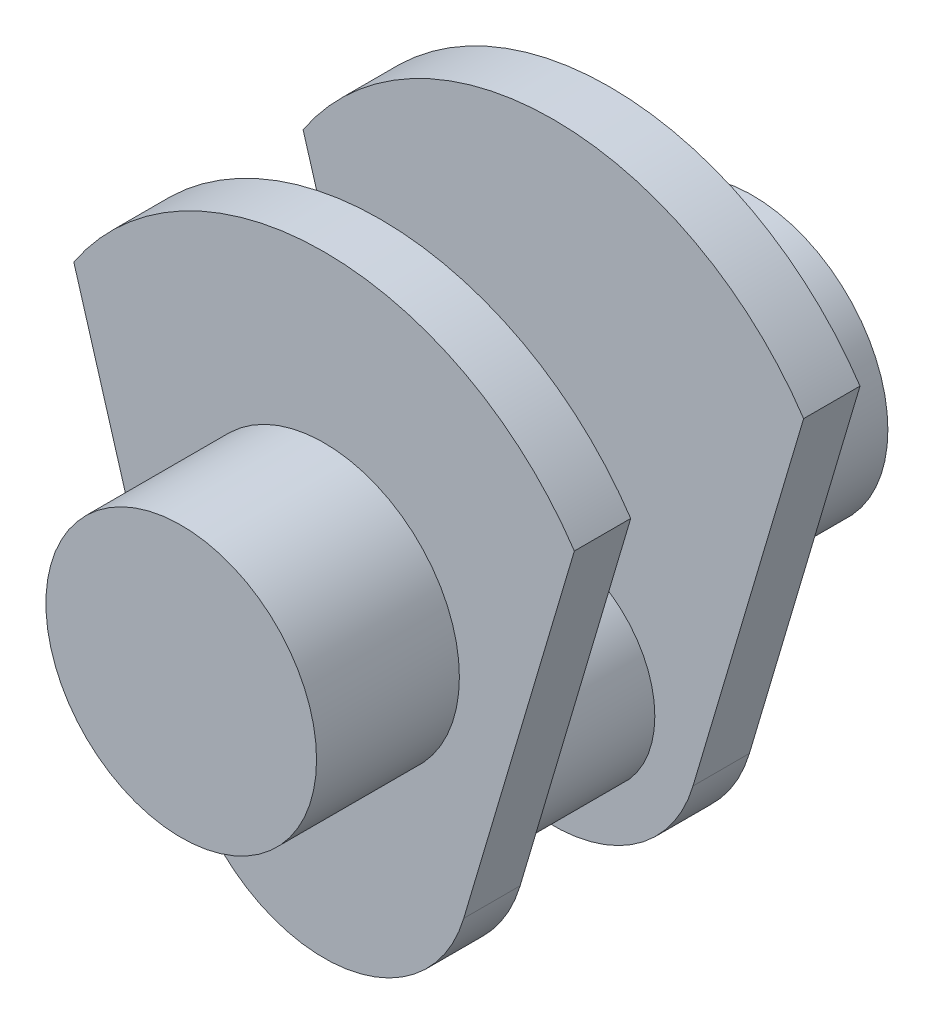
ISO-10303-21;
HEADER;
FILE_DESCRIPTION(('STEP AP214'),'2;1');
FILE_NAME('part.step','',(''),(''),'','','');
FILE_SCHEMA(('AUTOMOTIVE_DESIGN { 1 0 10303 214 1 1 1 1 }'));
ENDSEC;
DATA;
#1=APPLICATION_CONTEXT('core data for automotive mechanical design processes');
#2=APPLICATION_PROTOCOL_DEFINITION('international standard','automotive_design',2000,#1);
#3=PRODUCT_CONTEXT('',#1,'mechanical');
#4=PRODUCT('Part','Part','',(#3));
#5=PRODUCT_RELATED_PRODUCT_CATEGORY('part','',(#4));
#6=PRODUCT_DEFINITION_FORMATION('','',#4);
#7=PRODUCT_DEFINITION_CONTEXT('part definition',#1,'design');
#8=PRODUCT_DEFINITION('design','',#6,#7);
#9=PRODUCT_DEFINITION_SHAPE('','',#8);
#10=(LENGTH_UNIT() NAMED_UNIT(*) SI_UNIT(.MILLI.,.METRE.));
#11=(NAMED_UNIT(*) PLANE_ANGLE_UNIT() SI_UNIT($,.RADIAN.));
#12=(NAMED_UNIT(*) SI_UNIT($,.STERADIAN.) SOLID_ANGLE_UNIT());
#13=UNCERTAINTY_MEASURE_WITH_UNIT(LENGTH_MEASURE(1.E-05),#10,'distance_accuracy_value','');
#14=(GEOMETRIC_REPRESENTATION_CONTEXT(3) GLOBAL_UNCERTAINTY_ASSIGNED_CONTEXT((#13)) GLOBAL_UNIT_ASSIGNED_CONTEXT((#10,
#11,#12)) REPRESENTATION_CONTEXT('',''));
#15=CARTESIAN_POINT('',(0.,0.,0.));
#16=DIRECTION('',(0.,0.,1.));
#17=DIRECTION('',(1.,0.,0.));
#18=AXIS2_PLACEMENT_3D('',#15,#16,#17);
#19=CARTESIAN_POINT('',(0.,0.,15.));
#20=DIRECTION('',(0.,0.,-1.));
#21=DIRECTION('',(-1.,0.,0.));
#22=AXIS2_PLACEMENT_3D('',#19,#20,#21);
#23=CYLINDRICAL_SURFACE('',#22,80.);
#24=CARTESIAN_POINT('',(0.,0.,0.));
#25=DIRECTION('',(0.,0.,1.));
#26=DIRECTION('',(1.,0.,0.));
#27=AXIS2_PLACEMENT_3D('',#24,#25,#26);
#28=CIRCLE('',#27,80.);
#29=CARTESIAN_POINT('',(-66.5833173563063,44.3470613437846,0.));
#30=VERTEX_POINT('',#29);
#31=CARTESIAN_POINT('',(66.5833173563063,44.3470613437847,0.));
#32=VERTEX_POINT('',#31);
#33=EDGE_CURVE('E150',#30,#32,#28,.F.);
#34=ORIENTED_EDGE('',*,*,#33,.F.);
#35=DIRECTION('',(0.,0.,-1.));
#36=VECTOR('',#35,1.);
#37=CARTESIAN_POINT('',(-66.5833173563063,44.3470613437846,15.));
#38=LINE('',#37,#36);
#39=CARTESIAN_POINT('',(-66.5833173563063,44.3470613437846,15.));
#40=VERTEX_POINT('',#39);
#41=EDGE_CURVE('E84',#40,#30,#38,.T.);
#42=ORIENTED_EDGE('',*,*,#41,.F.);
#43=CARTESIAN_POINT('',(0.,0.,15.));
#44=DIRECTION('',(0.,0.,1.));
#45=DIRECTION('',(1.,0.,0.));
#46=AXIS2_PLACEMENT_3D('',#43,#44,#45);
#47=CIRCLE('',#46,80.);
#48=CARTESIAN_POINT('',(66.5833173563063,44.3470613437847,15.));
#49=VERTEX_POINT('',#48);
#50=EDGE_CURVE('E146',#40,#49,#47,.F.);
#51=ORIENTED_EDGE('',*,*,#50,.T.);
#52=DIRECTION('',(0.,0.,-1.));
#53=VECTOR('',#52,1.);
#54=CARTESIAN_POINT('',(66.5833173563063,44.3470613437847,15.));
#55=LINE('',#54,#53);
#56=EDGE_CURVE('E59',#49,#32,#55,.T.);
#57=ORIENTED_EDGE('',*,*,#56,.T.);
#58=EDGE_LOOP('',(#34,#42,#51,#57));
#59=FACE_BOUND('',#58,.T.);
#60=ADVANCED_FACE('F41',(#59),#23,.T.);
#61=CARTESIAN_POINT('',(-49.1358226215895,-14.5546937465779,15.));
#62=DIRECTION('',(0.958819734868193,0.284015344703923,0.));
#63=DIRECTION('',(-0.284015344703924,0.958819734868193,0.));
#64=AXIS2_PLACEMENT_3D('',#61,#62,#63);
#65=PLANE('',#64);
#66=DIRECTION('',(0.284015344703924,-0.958819734868193,0.));
#67=VECTOR('',#66,1.);
#68=CARTESIAN_POINT('',(-49.1358226215895,-14.5546937465779,0.));
#69=LINE('',#68,#67);
#70=CARTESIAN_POINT('',(-37.1537638512589,-55.0054462413772,0.));
#71=VERTEX_POINT('',#70);
#72=EDGE_CURVE('E158',#30,#71,#69,.T.);
#73=ORIENTED_EDGE('',*,*,#72,.T.);
#74=DIRECTION('',(0.,0.,-1.));
#75=VECTOR('',#74,1.);
#76=CARTESIAN_POINT('',(-37.1537638512589,-55.0054462413772,15.));
#77=LINE('',#76,#75);
#78=CARTESIAN_POINT('',(-37.1537638512589,-55.0054462413772,15.));
#79=VERTEX_POINT('',#78);
#80=EDGE_CURVE('E167',#79,#71,#77,.T.);
#81=ORIENTED_EDGE('',*,*,#80,.F.);
#82=DIRECTION('',(0.284015344703924,-0.958819734868193,0.));
#83=VECTOR('',#82,1.);
#84=CARTESIAN_POINT('',(-49.1358226215895,-14.5546937465779,15.));
#85=LINE('',#84,#83);
#86=EDGE_CURVE('E147',#40,#79,#85,.T.);
#87=ORIENTED_EDGE('',*,*,#86,.F.);
#88=ORIENTED_EDGE('',*,*,#41,.T.);
#89=EDGE_LOOP('',(#73,#81,#87,#88));
#90=FACE_BOUND('',#89,.T.);
#91=ADVANCED_FACE('F193',(#90),#65,.F.);
#92=CARTESIAN_POINT('',(0.,-44.,15.));
#93=DIRECTION('',(0.,0.,-1.));
#94=DIRECTION('',(-1.,0.,0.));
#95=AXIS2_PLACEMENT_3D('',#92,#93,#94);
#96=CYLINDRICAL_SURFACE('',#95,38.7494776130847);
#97=CARTESIAN_POINT('',(0.,-44.,0.));
#98=DIRECTION('',(0.,0.,1.));
#99=DIRECTION('',(1.,0.,0.));
#100=AXIS2_PLACEMENT_3D('',#97,#98,#99);
#101=CIRCLE('',#100,38.7494776130847);
#102=CARTESIAN_POINT('',(37.1537638512589,-55.0054462413772,0.));
#103=VERTEX_POINT('',#102);
#104=EDGE_CURVE('E159',#71,#103,#101,.T.);
#105=ORIENTED_EDGE('',*,*,#104,.T.);
#106=DIRECTION('',(0.,0.,-1.));
#107=VECTOR('',#106,1.);
#108=CARTESIAN_POINT('',(37.1537638512589,-55.0054462413772,15.));
#109=LINE('',#108,#107);
#110=CARTESIAN_POINT('',(37.1537638512589,-55.0054462413772,15.));
#111=VERTEX_POINT('',#110);
#112=EDGE_CURVE('E74',#111,#103,#109,.T.);
#113=ORIENTED_EDGE('',*,*,#112,.F.);
#114=CARTESIAN_POINT('',(0.,-44.,15.));
#115=DIRECTION('',(0.,0.,1.));
#116=DIRECTION('',(1.,0.,0.));
#117=AXIS2_PLACEMENT_3D('',#114,#115,#116);
#118=CIRCLE('',#117,38.7494776130847);
#119=EDGE_CURVE('E153',#79,#111,#118,.T.);
#120=ORIENTED_EDGE('',*,*,#119,.F.);
#121=ORIENTED_EDGE('',*,*,#80,.T.);
#122=EDGE_LOOP('',(#105,#113,#120,#121));
#123=FACE_BOUND('',#122,.T.);
#124=ADVANCED_FACE('F181',(#123),#96,.T.);
#125=CARTESIAN_POINT('',(49.1358226215895,-14.5546937465779,15.));
#126=DIRECTION('',(0.958819734868193,-0.284015344703923,0.));
#127=DIRECTION('',(0.284015344703923,0.958819734868193,0.));
#128=AXIS2_PLACEMENT_3D('',#125,#126,#127);
#129=PLANE('',#128);
#130=DIRECTION('',(-0.284015344703923,-0.958819734868193,0.));
#131=VECTOR('',#130,1.);
#132=CARTESIAN_POINT('',(49.1358226215895,-14.5546937465779,0.));
#133=LINE('',#132,#131);
#134=EDGE_CURVE('E151',#32,#103,#133,.T.);
#135=ORIENTED_EDGE('',*,*,#134,.F.);
#136=ORIENTED_EDGE('',*,*,#56,.F.);
#137=DIRECTION('',(-0.284015344703923,-0.958819734868193,0.));
#138=VECTOR('',#137,1.);
#139=CARTESIAN_POINT('',(49.1358226215895,-14.5546937465779,15.));
#140=LINE('',#139,#138);
#141=EDGE_CURVE('E154',#49,#111,#140,.T.);
#142=ORIENTED_EDGE('',*,*,#141,.T.);
#143=ORIENTED_EDGE('',*,*,#112,.T.);
#144=EDGE_LOOP('',(#135,#136,#142,#143));
#145=FACE_BOUND('',#144,.T.);
#146=ADVANCED_FACE('F182',(#145),#129,.T.);
#147=CARTESIAN_POINT('',(0.,0.,15.));
#148=DIRECTION('',(0.,0.,1.));
#149=DIRECTION('',(1.,0.,0.));
#150=AXIS2_PLACEMENT_3D('',#147,#148,#149);
#151=PLANE('',#150);
#152=CARTESIAN_POINT('',(0.,0.,15.));
#153=DIRECTION('',(0.,0.,1.));
#154=DIRECTION('',(1.,0.,0.));
#155=AXIS2_PLACEMENT_3D('',#152,#153,#154);
#156=CIRCLE('',#155,36.);
#157=CARTESIAN_POINT('',(36.,0.,15.));
#158=VERTEX_POINT('',#157);
#159=EDGE_CURVE('E11',#158,#158,#156,.T.);
#160=ORIENTED_EDGE('',*,*,#159,.F.);
#161=EDGE_LOOP('',(#160));
#162=FACE_BOUND('',#161,.T.);
#163=ORIENTED_EDGE('',*,*,#50,.F.);
#164=ORIENTED_EDGE('',*,*,#86,.T.);
#165=ORIENTED_EDGE('',*,*,#119,.T.);
#166=ORIENTED_EDGE('',*,*,#141,.F.);
#167=EDGE_LOOP('',(#163,#164,#165,#166));
#168=FACE_BOUND('',#167,.T.);
#169=ADVANCED_FACE('F177',(#162,#168),#151,.T.);
#170=CARTESIAN_POINT('',(0.,0.,0.));
#171=DIRECTION('',(0.,0.,1.));
#172=DIRECTION('',(1.,0.,0.));
#173=AXIS2_PLACEMENT_3D('',#170,#171,#172);
#174=PLANE('',#173);
#175=CARTESIAN_POINT('',(0.,-44.,0.));
#176=DIRECTION('',(0.,0.,1.));
#177=DIRECTION('',(1.,0.,0.));
#178=AXIS2_PLACEMENT_3D('',#175,#176,#177);
#179=CIRCLE('',#178,27.);
#180=CARTESIAN_POINT('',(27.,-44.,0.));
#181=VERTEX_POINT('',#180);
#182=EDGE_CURVE('E42',#181,#181,#179,.F.);
#183=ORIENTED_EDGE('',*,*,#182,.F.);
#184=EDGE_LOOP('',(#183));
#185=FACE_BOUND('',#184,.T.);
#186=ORIENTED_EDGE('',*,*,#33,.T.);
#187=ORIENTED_EDGE('',*,*,#134,.T.);
#188=ORIENTED_EDGE('',*,*,#104,.F.);
#189=ORIENTED_EDGE('',*,*,#72,.F.);
#190=EDGE_LOOP('',(#186,#187,#188,#189));
#191=FACE_BOUND('',#190,.T.);
#192=ADVANCED_FACE('F175',(#185,#191),#174,.F.);
#193=CARTESIAN_POINT('',(0.,-44.,-46.));
#194=DIRECTION('',(0.,0.,1.));
#195=DIRECTION('',(1.,0.,0.));
#196=AXIS2_PLACEMENT_3D('',#193,#194,#195);
#197=CYLINDRICAL_SURFACE('',#196,27.);
#198=CARTESIAN_POINT('',(0.,-44.,-46.));
#199=DIRECTION('',(0.,0.,-1.));
#200=DIRECTION('',(-1.,0.,0.));
#201=AXIS2_PLACEMENT_3D('',#198,#199,#200);
#202=CIRCLE('',#201,27.);
#203=CARTESIAN_POINT('',(-27.,-44.,-46.));
#204=VERTEX_POINT('',#203);
#205=EDGE_CURVE('E140',#204,#204,#202,.T.);
#206=ORIENTED_EDGE('',*,*,#205,.F.);
#207=EDGE_LOOP('',(#206));
#208=FACE_BOUND('',#207,.T.);
#209=ORIENTED_EDGE('',*,*,#182,.T.);
#210=EDGE_LOOP('',(#209));
#211=FACE_BOUND('',#210,.T.);
#212=ADVANCED_FACE('F174',(#208,#211),#197,.T.);
#213=CARTESIAN_POINT('',(0.,0.,53.));
#214=DIRECTION('',(0.,0.,-1.));
#215=DIRECTION('',(-1.,0.,0.));
#216=AXIS2_PLACEMENT_3D('',#213,#214,#215);
#217=CYLINDRICAL_SURFACE('',#216,36.);
#218=CARTESIAN_POINT('',(0.,0.,53.));
#219=DIRECTION('',(0.,0.,1.));
#220=DIRECTION('',(1.,0.,0.));
#221=AXIS2_PLACEMENT_3D('',#218,#219,#220);
#222=CIRCLE('',#221,36.);
#223=CARTESIAN_POINT('',(36.,0.,53.));
#224=VERTEX_POINT('',#223);
#225=EDGE_CURVE('E138',#224,#224,#222,.T.);
#226=ORIENTED_EDGE('',*,*,#225,.F.);
#227=EDGE_LOOP('',(#226));
#228=FACE_BOUND('',#227,.T.);
#229=ORIENTED_EDGE('',*,*,#159,.T.);
#230=EDGE_LOOP('',(#229));
#231=FACE_BOUND('',#230,.T.);
#232=ADVANCED_FACE('F244',(#228,#231),#217,.T.);
#233=CARTESIAN_POINT('',(0.,0.,53.));
#234=DIRECTION('',(0.,0.,1.));
#235=DIRECTION('',(1.,0.,0.));
#236=AXIS2_PLACEMENT_3D('',#233,#234,#235);
#237=PLANE('',#236);
#238=ORIENTED_EDGE('',*,*,#225,.T.);
#239=EDGE_LOOP('',(#238));
#240=FACE_BOUND('',#239,.T.);
#241=ADVANCED_FACE('F252',(#240),#237,.T.);
#242=CARTESIAN_POINT('',(0.,0.,-61.));
#243=DIRECTION('',(0.,0.,1.));
#244=DIRECTION('',(1.,0.,0.));
#245=AXIS2_PLACEMENT_3D('',#242,#243,#244);
#246=CYLINDRICAL_SURFACE('',#245,80.);
#247=CARTESIAN_POINT('',(0.,0.,-46.));
#248=DIRECTION('',(0.,0.,1.));
#249=DIRECTION('',(1.,0.,0.));
#250=AXIS2_PLACEMENT_3D('',#247,#248,#249);
#251=CIRCLE('',#250,80.);
#252=CARTESIAN_POINT('',(-66.5833173563063,44.3470613437846,-46.));
#253=VERTEX_POINT('',#252);
#254=CARTESIAN_POINT('',(66.5833173563063,44.3470613437847,-46.));
#255=VERTEX_POINT('',#254);
#256=EDGE_CURVE('E135',#253,#255,#251,.F.);
#257=ORIENTED_EDGE('',*,*,#256,.T.);
#258=DIRECTION('',(0.,0.,1.));
#259=VECTOR('',#258,1.);
#260=CARTESIAN_POINT('',(66.5833173563063,44.3470613437847,-61.));
#261=LINE('',#260,#259);
#262=CARTESIAN_POINT('',(66.5833173563063,44.3470613437847,-61.));
#263=VERTEX_POINT('',#262);
#264=EDGE_CURVE('E116',#263,#255,#261,.T.);
#265=ORIENTED_EDGE('',*,*,#264,.F.);
#266=CARTESIAN_POINT('',(0.,0.,-61.));
#267=DIRECTION('',(0.,0.,1.));
#268=DIRECTION('',(1.,0.,0.));
#269=AXIS2_PLACEMENT_3D('',#266,#267,#268);
#270=CIRCLE('',#269,80.);
#271=CARTESIAN_POINT('',(-66.5833173563063,44.3470613437846,-61.));
#272=VERTEX_POINT('',#271);
#273=EDGE_CURVE('E122',#272,#263,#270,.F.);
#274=ORIENTED_EDGE('',*,*,#273,.F.);
#275=DIRECTION('',(0.,0.,1.));
#276=VECTOR('',#275,1.);
#277=CARTESIAN_POINT('',(-66.5833173563063,44.3470613437846,-61.));
#278=LINE('',#277,#276);
#279=EDGE_CURVE('E359',#272,#253,#278,.T.);
#280=ORIENTED_EDGE('',*,*,#279,.T.);
#281=EDGE_LOOP('',(#257,#265,#274,#280));
#282=FACE_BOUND('',#281,.T.);
#283=ADVANCED_FACE('F134',(#282),#246,.T.);
#284=CARTESIAN_POINT('',(49.1358226215895,-14.5546937465779,-61.));
#285=DIRECTION('',(-0.958819734868193,0.284015344703923,0.));
#286=DIRECTION('',(-0.284015344703923,-0.958819734868193,0.));
#287=AXIS2_PLACEMENT_3D('',#284,#285,#286);
#288=PLANE('',#287);
#289=DIRECTION('',(-0.284015344703923,-0.958819734868193,0.));
#290=VECTOR('',#289,1.);
#291=CARTESIAN_POINT('',(49.1358226215895,-14.5546937465779,-46.));
#292=LINE('',#291,#290);
#293=CARTESIAN_POINT('',(37.1537638512589,-55.0054462413772,-46.));
#294=VERTEX_POINT('',#293);
#295=EDGE_CURVE('E351',#255,#294,#292,.T.);
#296=ORIENTED_EDGE('',*,*,#295,.T.);
#297=DIRECTION('',(0.,0.,1.));
#298=VECTOR('',#297,1.);
#299=CARTESIAN_POINT('',(37.1537638512589,-55.0054462413772,-61.));
#300=LINE('',#299,#298);
#301=CARTESIAN_POINT('',(37.1537638512589,-55.0054462413772,-61.));
#302=VERTEX_POINT('',#301);
#303=EDGE_CURVE('E119',#302,#294,#300,.T.);
#304=ORIENTED_EDGE('',*,*,#303,.F.);
#305=DIRECTION('',(-0.284015344703923,-0.958819734868193,0.));
#306=VECTOR('',#305,1.);
#307=CARTESIAN_POINT('',(49.1358226215895,-14.5546937465779,-61.));
#308=LINE('',#307,#306);
#309=EDGE_CURVE('E112',#263,#302,#308,.T.);
#310=ORIENTED_EDGE('',*,*,#309,.F.);
#311=ORIENTED_EDGE('',*,*,#264,.T.);
#312=EDGE_LOOP('',(#296,#304,#310,#311));
#313=FACE_BOUND('',#312,.T.);
#314=ADVANCED_FACE('F111',(#313),#288,.F.);
#315=CARTESIAN_POINT('',(0.,-44.,-61.));
#316=DIRECTION('',(0.,0.,1.));
#317=DIRECTION('',(1.,0.,0.));
#318=AXIS2_PLACEMENT_3D('',#315,#316,#317);
#319=CYLINDRICAL_SURFACE('',#318,38.7494776130847);
#320=CARTESIAN_POINT('',(0.,-44.,-46.));
#321=DIRECTION('',(0.,0.,1.));
#322=DIRECTION('',(1.,0.,0.));
#323=AXIS2_PLACEMENT_3D('',#320,#321,#322);
#324=CIRCLE('',#323,38.7494776130847);
#325=CARTESIAN_POINT('',(-37.1537638512589,-55.0054462413772,-46.));
#326=VERTEX_POINT('',#325);
#327=EDGE_CURVE('E356',#326,#294,#324,.T.);
#328=ORIENTED_EDGE('',*,*,#327,.F.);
#329=DIRECTION('',(0.,0.,1.));
#330=VECTOR('',#329,1.);
#331=CARTESIAN_POINT('',(-37.1537638512589,-55.0054462413772,-61.));
#332=LINE('',#331,#330);
#333=CARTESIAN_POINT('',(-37.1537638512589,-55.0054462413772,-61.));
#334=VERTEX_POINT('',#333);
#335=EDGE_CURVE('E143',#334,#326,#332,.T.);
#336=ORIENTED_EDGE('',*,*,#335,.F.);
#337=CARTESIAN_POINT('',(0.,-44.,-61.));
#338=DIRECTION('',(0.,0.,1.));
#339=DIRECTION('',(1.,0.,0.));
#340=AXIS2_PLACEMENT_3D('',#337,#338,#339);
#341=CIRCLE('',#340,38.7494776130847);
#342=EDGE_CURVE('E124',#334,#302,#341,.T.);
#343=ORIENTED_EDGE('',*,*,#342,.T.);
#344=ORIENTED_EDGE('',*,*,#303,.T.);
#345=EDGE_LOOP('',(#328,#336,#343,#344));
#346=FACE_BOUND('',#345,.T.);
#347=ADVANCED_FACE('F276',(#346),#319,.T.);
#348=CARTESIAN_POINT('',(-49.1358226215895,-14.5546937465779,-61.));
#349=DIRECTION('',(-0.958819734868193,-0.284015344703923,0.));
#350=DIRECTION('',(0.284015344703924,-0.958819734868193,0.));
#351=AXIS2_PLACEMENT_3D('',#348,#349,#350);
#352=PLANE('',#351);
#353=DIRECTION('',(0.284015344703924,-0.958819734868193,0.));
#354=VECTOR('',#353,1.);
#355=CARTESIAN_POINT('',(-49.1358226215895,-14.5546937465779,-46.));
#356=LINE('',#355,#354);
#357=EDGE_CURVE('E131',#253,#326,#356,.T.);
#358=ORIENTED_EDGE('',*,*,#357,.F.);
#359=ORIENTED_EDGE('',*,*,#279,.F.);
#360=DIRECTION('',(0.284015344703924,-0.958819734868193,0.));
#361=VECTOR('',#360,1.);
#362=CARTESIAN_POINT('',(-49.1358226215895,-14.5546937465779,-61.));
#363=LINE('',#362,#361);
#364=EDGE_CURVE('E129',#272,#334,#363,.T.);
#365=ORIENTED_EDGE('',*,*,#364,.T.);
#366=ORIENTED_EDGE('',*,*,#335,.T.);
#367=EDGE_LOOP('',(#358,#359,#365,#366));
#368=FACE_BOUND('',#367,.T.);
#369=ADVANCED_FACE('F287',(#368),#352,.T.);
#370=CARTESIAN_POINT('',(0.,0.,-61.));
#371=DIRECTION('',(0.,0.,-1.));
#372=DIRECTION('',(1.,0.,0.));
#373=AXIS2_PLACEMENT_3D('',#370,#371,#372);
#374=PLANE('',#373);
#375=CARTESIAN_POINT('',(0.,0.,-61.));
#376=DIRECTION('',(0.,0.,1.));
#377=DIRECTION('',(1.,0.,0.));
#378=AXIS2_PLACEMENT_3D('',#375,#376,#377);
#379=CIRCLE('',#378,36.);
#380=CARTESIAN_POINT('',(36.,0.,-61.));
#381=VERTEX_POINT('',#380);
#382=EDGE_CURVE('E349',#381,#381,#379,.T.);
#383=ORIENTED_EDGE('',*,*,#382,.T.);
#384=EDGE_LOOP('',(#383));
#385=FACE_BOUND('',#384,.T.);
#386=ORIENTED_EDGE('',*,*,#273,.T.);
#387=ORIENTED_EDGE('',*,*,#309,.T.);
#388=ORIENTED_EDGE('',*,*,#342,.F.);
#389=ORIENTED_EDGE('',*,*,#364,.F.);
#390=EDGE_LOOP('',(#386,#387,#388,#389));
#391=FACE_BOUND('',#390,.T.);
#392=ADVANCED_FACE('F130',(#385,#391),#374,.T.);
#393=CARTESIAN_POINT('',(0.,0.,-46.));
#394=DIRECTION('',(0.,0.,-1.));
#395=DIRECTION('',(1.,0.,0.));
#396=AXIS2_PLACEMENT_3D('',#393,#394,#395);
#397=PLANE('',#396);
#398=ORIENTED_EDGE('',*,*,#205,.T.);
#399=EDGE_LOOP('',(#398));
#400=FACE_BOUND('',#399,.T.);
#401=ORIENTED_EDGE('',*,*,#256,.F.);
#402=ORIENTED_EDGE('',*,*,#357,.T.);
#403=ORIENTED_EDGE('',*,*,#327,.T.);
#404=ORIENTED_EDGE('',*,*,#295,.F.);
#405=EDGE_LOOP('',(#401,#402,#403,#404));
#406=FACE_BOUND('',#405,.T.);
#407=ADVANCED_FACE('F307',(#400,#406),#397,.F.);
#408=CARTESIAN_POINT('',(0.,0.,-99.));
#409=DIRECTION('',(0.,0.,1.));
#410=DIRECTION('',(1.,0.,0.));
#411=AXIS2_PLACEMENT_3D('',#408,#409,#410);
#412=CYLINDRICAL_SURFACE('',#411,36.);
#413=CARTESIAN_POINT('',(0.,0.,-99.));
#414=DIRECTION('',(0.,0.,1.));
#415=DIRECTION('',(1.,0.,0.));
#416=AXIS2_PLACEMENT_3D('',#413,#414,#415);
#417=CIRCLE('',#416,36.);
#418=CARTESIAN_POINT('',(36.,0.,-99.));
#419=VERTEX_POINT('',#418);
#420=EDGE_CURVE('E346',#419,#419,#417,.T.);
#421=ORIENTED_EDGE('',*,*,#420,.T.);
#422=EDGE_LOOP('',(#421));
#423=FACE_BOUND('',#422,.T.);
#424=ORIENTED_EDGE('',*,*,#382,.F.);
#425=EDGE_LOOP('',(#424));
#426=FACE_BOUND('',#425,.T.);
#427=ADVANCED_FACE('F319',(#423,#426),#412,.T.);
#428=CARTESIAN_POINT('',(0.,0.,-99.));
#429=DIRECTION('',(0.,0.,-1.));
#430=DIRECTION('',(1.,0.,0.));
#431=AXIS2_PLACEMENT_3D('',#428,#429,#430);
#432=PLANE('',#431);
#433=ORIENTED_EDGE('',*,*,#420,.F.);
#434=EDGE_LOOP('',(#433));
#435=FACE_BOUND('',#434,.T.);
#436=ADVANCED_FACE('F334',(#435),#432,.T.);
#437=CLOSED_SHELL('',(#60,#91,#124,#146,#169,#192,#212,#232,#241,#283,#314,#347,#369,#392,#407,
#427,#436));
#438=MANIFOLD_SOLID_BREP('B2',#437);
#439=ADVANCED_BREP_SHAPE_REPRESENTATION('',(#18,#438),#14);
#440=SHAPE_DEFINITION_REPRESENTATION(#9,#439);
ENDSEC;
END-ISO-10303-21;
